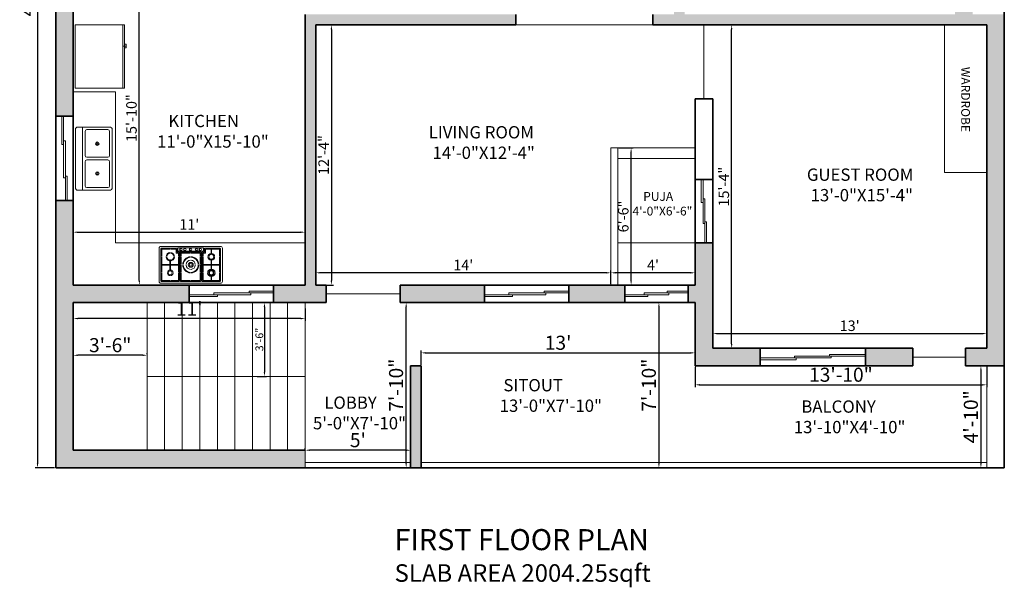
# Model space of a CAD drawing. Units: inches. Extents: x 3491 to 6898, y 1360 to 2019.
# Tile 8 of 9: x 6321 to 6882, y 1360 to 1683. Entities that reach past the tile are written whole.
import ezdxf

# ---------------------------------------------------------------- set-up
doc = ezdxf.new("R2010")
doc.units = ezdxf.units.IN
for name, color, linetype, lineweight in [('A-ANNO-DIMS', 2, 'Continuous', 18), ('A-ANNO-TEXT', 7, 'Continuous', 18), ('A-ANNO-TITL', 7, 'Continuous', 30), ('A-AREA-IDEN', 7, 'Continuous', 18), ('A-DOOR', 4, 'Continuous', 18), ('A-EQPM', 8, 'Continuous', 18), ('A-FLOR-CASE', 8, 'Continuous', 18), ('A-FLOR-FIXT', 8, 'Continuous', 18), ('A-FLOR-RAL', 7, 'Continuous', 18), ('A-FLOR-STRS', 7, 'Continuous', 18), ('A-GLAZ', 5, 'Continuous', 18), ('A-WALL', 7, 'Continuous', 35), ('A-WALL-PATT', 8, 'Continuous', 13)]:
    doc.layers.add(name, color=color, linetype=linetype, lineweight=lineweight)
doc.layers.add('A-WALL-OPEN', color=251, linetype='Continuous', lineweight=13, true_color=0x636466)
doc.styles.get("Standard").update_dxf_attribs({"font": 'arial.ttf'})
doc.dimstyles.new('ISO-25', dxfattribs={"dimtxt": 8, "dimasz": 2.5, "dimexe": 1.25, "dimexo": 0.625, "dimtad": 1, "dimdec": 1, "dimlunit": 3, "dimtxsty": 'Standard', "dimcen": 2.5, "dimclrt": 1, "dimadec": 0, "dimazin": 0, "dimtfac": 1, "dimtdec": 1, "dimtmove": 0, "dimatfit": 3, "dimfxl": 1, "dimarcsym": 0})

# ---------------------------------------------------------------- blocks, each defined once
blk = doc.blocks.new('*D35')
at = {"layer": 'A-ANNO-DIMS', "color": 0, "lineweight": -2, "transparency": 16777216}
for p, q in [((6341.16, 1972.37), (6330.15, 1972.37)), ((6331.4, 1969.87), (6331.4, 1430.87)), ((6341.16, 1428.37), (6330.15, 1428.37))]:
    blk.add_line(p, q, dxfattribs=at)
at = {"layer": 'A-ANNO-DIMS', "color": 0, "transparency": 16777216}
for points in [[(6330.99, 1969.87), (6331.82, 1969.87), (6331.4, 1972.37)], [(6330.99, 1430.87), (6331.82, 1430.87), (6331.4, 1428.37)]]:
    blk.add_solid(points, dxfattribs=at)
at = {"layer": 'Defpoints', "color": 0, "transparency": 16777216}
for p in [(6341.78, 1972.37), (6331.4, 1428.37), (6341.78, 1428.37)]:
    blk.add_point(p, dxfattribs=at)
at = {"layer": 'A-ANNO-DIMS', "color": 0, "transparency": 16777216, "insert": (6326.71, 1700.37), "char_height": 8, "attachment_point": 5, "rotation": 90}
blk.add_mtext('45\'-4"', dxfattribs=at)
blk = doc.blocks.new('*D36')
at = {"layer": 'A-ANNO-DIMS', "color": 0, "lineweight": -2, "transparency": 16777216}
for p, q in [((6351.78, 1493.03), (6351.78, 1493.65)), ((6391.28, 1492.4), (6354.28, 1492.4)), ((6393.78, 1493.03), (6393.78, 1493.65))]:
    blk.add_line(p, q, dxfattribs=at)
at = {"layer": 'A-ANNO-DIMS', "color": 0, "transparency": 16777216}
for points in [[(6354.28, 1492.82), (6354.28, 1491.99), (6351.78, 1492.4)], [(6391.28, 1492.82), (6391.28, 1491.99), (6393.78, 1492.4)]]:
    blk.add_solid(points, dxfattribs=at)
at = {"layer": 'Defpoints', "color": 0, "transparency": 16777216}
for p in [(6351.78, 1492.4), (6351.78, 1492.4), (6393.78, 1492.4)]:
    blk.add_point(p, dxfattribs=at)
at = {"layer": 'A-ANNO-DIMS', "color": 0, "transparency": 16777216, "insert": (6372.78, 1497.12), "char_height": 8, "attachment_point": 5}
blk.add_mtext('3\'-6"', dxfattribs=at)
blk = doc.blocks.new('*D30')
at = {"layer": 'A-ANNO-DIMS', "color": 0, "lineweight": -2, "transparency": 16777216}
for p, q in [((6456.5, 1522.37), (6461.84, 1522.37)), ((6460.59, 1519.87), (6460.59, 1482.87)), ((6456.5, 1480.37), (6461.84, 1480.37))]:
    blk.add_line(p, q, dxfattribs=at)
at = {"layer": 'A-ANNO-DIMS', "color": 0, "transparency": 16777216}
for points in [[(6460.17, 1519.87), (6461.01, 1519.87), (6460.59, 1522.37)], [(6460.17, 1482.87), (6461.01, 1482.87), (6460.59, 1480.37)]]:
    blk.add_solid(points, dxfattribs=at)
at = {"layer": 'Defpoints', "color": 0, "transparency": 16777216}
for p in [(6455.87, 1522.37), (6455.87, 1480.37), (6460.59, 1480.37)]:
    blk.add_point(p, dxfattribs=at)
at = {"layer": 'A-ANNO-DIMS', "color": 0, "transparency": 16777216, "insert": (6457.69, 1501.37), "char_height": 8, "attachment_point": 5, "rotation": 90}
blk.add_mtext('{\\H0.55556x;3\'-6"}', dxfattribs=at)
blk = doc.blocks.new('STOVE')
for p, q in [((11.85, 19.7), (11.55, 19.7)), ((11.55, 16.92), (11.55, 19.7)), ((11.85, 16.92), (11.55, 16.92)), ((11.85, 16.92), (11.85, 19.7)), ((-11.85, 13.73), (-11.85, 7.62)), ((-11.85, 13.73), (-11.55, 13.73)), ((-11.55, 13.73), (-11.55, 7.62)), ((11.85, 13.23), (11.55, 13.23)), ((11.55, 13.23), (11.55, 7.57)), ((11.85, 13.23), (11.85, 7.57)), ((-11.85, 10.75), (-16.4, 10.75)), ((-11.85, 10.25), (-16.4, 10.25)), ((-11.85, 7.62), (-11.55, 7.62)), ((-7, 10.75), (-11.55, 10.75)), ((-7, 10.25), (-11.55, 10.25)), ((7, 10.75), (11.55, 10.75)), ((7, 10.25), (11.55, 10.25)), ((11.85, 7.57), (11.55, 7.57)), ((11.85, 10.75), (16.4, 10.75)), ((11.85, 10.25), (16.4, 10.25)), ((-7, 3.9), (-8.4, 3.9)), ((-7.8, 3.3), (-7.8, 1)), ((-6.4, 3.3), (-7.8, 3.3)), ((7.3, 2.8), (-7.3, 2.8)), ((-7.3, 2.8), (-7.3, 0.8)), ((7.3, 0.8), (-7.3, 0.8)), ((-5.4, 3.9), (-6, 3.9)), ((-5.4, 3.9), (-0.15, 3.9)), ((0.15, 3.9), (5.4, 3.9)), ((6.4, 3.3), (7.8, 3.3)), ((7, 3.9), (8.4, 3.9)), ((7.3, 2.8), (7.3, 0.8)), ((7.8, 3.3), (7.8, 1)), ((8.4, 3.9), (8.4, 1.6)), ((11.85, 4.28), (11.55, 4.28)), ((11.55, 4.28), (11.55, 1.3)), ((11.85, 1.3), (11.55, 1.3)), ((11.85, 4.28), (11.85, 1.3))]:
    blk.add_line(p, q)
for points in [[(-17, 21), (17, 21, -0.414214), (18, 20), (18, 1, -0.414214), (17, 0), (-17, 0, -0.414214), (-18, 1), (-18, 20, -0.414214)], [(6, 3.3), (-6, 3.3), (-6, 19.4, -0.414214), (-5.4, 20), (5.4, 20, -0.414214), (6, 19.4)]]:
    blk.add_lwpolyline(points, format="xyb", close=True)
for points in [[(-7.8, 1), (-16.4, 1, -0.414214), (-17, 1.6), (-17, 19.4, -0.414214), (-16.4, 20), (-7, 20, -0.414214), (-6.4, 19.4), (-6.4, 3.3)], [(6.4, 19.4, -0.414214), (7, 20), (16.4, 20, -0.414214), (17, 19.4), (17, 1.6, -0.414214), (16.4, 1), (7.8, 1)]]:
    blk.add_lwpolyline(points, format="xyb")
for points in [[(-16.4, 15.22), (-16.4, 19.4), (-11.85, 19.4)], [(-11.55, 19.4), (-7, 19.4), (-7, 15.22)], [(-5.4, 15.22), (-5.4, 19.4), (-0.15, 19.4)], [(0.15, 19.4), (5.4, 19.4), (5.4, 15.22)], [(6.4, 3.3), (6.4, 19.4)], [(7, 15.22), (7, 19.4), (11.55, 19.4)], [(11.85, 19.4), (16.4, 19.4), (16.4, 15.22)], [(-16.4, 6.08), (-16.4, 14.92)], [(-7, 14.92), (-7, 6.08)], [(-5.4, 10.65), (-5.4, 14.92)], [(5.4, 14.92), (5.4, 10.65)], [(7, 6.08), (7, 14.92)], [(16.4, 14.92), (16.4, 6.08)], [(-11.85, 1.6), (-16.4, 1.6), (-16.4, 5.77)], [(-7, 5.77), (-7, 3.9)], [(-5.4, 6.08), (-5.4, 10.35)], [(-5.4, 3.9), (-5.4, 5.77)], [(5.4, 10.35), (5.4, 6.08)], [(5.4, 5.77), (5.4, 3.9)], [(7, 3.9), (7, 5.77)], [(16.4, 5.77), (16.4, 1.6), (11.85, 1.6)], [(-8.4, 3.9), (-8.4, 1.6), (-11.55, 1.6)], [(11.55, 1.6), (8.4, 1.6)]]:
    blk.add_lwpolyline(points)
for centre, radius in [((-11.7, 15.07), 1.1), ((0, 10.5), 1.4), ((0, 10.5), 0.8), ((11.7, 15.07), 1.6), ((11.7, 15.07), 1.1), ((11.7, 5.93), 1.4), ((-5.49, 1.8), 0.6), ((-3.3, 1.8), 0.6), ((0, 1.8), 0.6), ((3.39, 1.8), 0.6), ((5.57, 1.8), 0.6)]:
    blk.add_circle(centre, radius)
for centre, radius, start, end in [((11.7, 15.07), 2.1, 94.096, 175.904), ((11.7, 15.07), 2.1, 4.096, 85.904), ((-11.7, 15.07), 1.6, 95.3794, 174.6206), ((-11.7, 15.07), 1.6, 185.3794, 264.6206), ((-11.7, 15.07), 1.6, 5.3794, 84.6206), ((-11.7, 15.07), 1.6, 275.3794, 354.6206), ((0, 10.5), 4.6, 91.8687, 178.1313), ((0, 10.5), 4.3, 91.9991, 178.0009), ((0, 10.5), 2.6, 93.3074, 176.6926), ((0, 10.5), 4.6, 1.8687, 88.1313), ((0, 10.5), 4.3, 1.9991, 88.0009), ((0, 10.5), 2.6, 3.3074, 86.6926), ((11.7, 15.07), 2.1, 184.096, 265.904), ((11.7, 15.07), 2.1, 274.096, 355.904), ((-11.7, 5.93), 2.4, 93.5833, 176.4167), ((-11.7, 5.93), 2.4, 183.5833, 266.4167), ((-11.7, 5.93), 2, 94.3012, 175.6988), ((-11.7, 5.93), 2, 184.3012, 265.6988), ((-11.7, 5.93), 2.4, 3.5833, 86.4167), ((-11.7, 5.93), 2, 4.3012, 85.6988), ((-11.7, 5.93), 2.4, 273.5833, 356.4167), ((-11.7, 5.93), 2, 274.3012, 355.6988), ((0, 10.5), 4.6, 181.8687, 268.1313), ((0, 10.5), 4.3, 181.9991, 268.0009), ((0, 10.5), 2.6, 183.3074, 266.6926), ((0, 10.5), 4.6, 271.8687, 358.1313), ((0, 10.5), 4.3, 271.9991, 358.0009), ((0, 10.5), 2.6, 273.3074, 356.6926), ((11.7, 5.93), 1.9, 94.5281, 175.4719), ((11.7, 5.93), 1.9, 184.5281, 265.4719), ((11.7, 5.93), 1.9, 4.5281, 85.4719), ((11.7, 5.93), 1.9, 274.5281, 355.4719), ((-5.49, 1.8), 0.846, 89.9979, 270), ((-3.3, 1.8), 0.846, 89.9979, 270), ((0, 1.8), 0.846, 89.9979, 270), ((3.39, 1.8), 0.846, 89.9979, 270), ((5.57, 1.8), 0.846, 89.9979, 270)]:
    blk.add_arc(centre, radius, start, end)
blk = doc.blocks.new('Sink-double - 36 in top')
for p, q in [((-18, -4), (18, -4)), ((-0.75, -18.5), (-0.75, -6.5)), ((0.75, -6.5), (0.75, -18.5))]:
    blk.add_line(p, q)
for points in [[(-16.5, 0), (16.5, 0)], [(-18, -19.5), (-18, -1.5)], [(-15.5, -5.5), (-1.75, -5.5)], [(1.75, -5.5), (15.5, -5.5)], [(18, -1.5), (18, -19.5)], [(-16.5, -18.5), (-16.5, -6.5)], [(16.5, -6.5), (16.5, -18.5)], [(16.5, -21), (-16.5, -21)], [(-1.75, -19.5), (-15.5, -19.5)], [(15.5, -19.5), (1.75, -19.5)]]:
    blk.add_lwpolyline(points)
for centre, radius in [((-8.5, -12.5), 1), ((-8.5, -12.5), 0.5), ((8.5, -12.5), 1), ((8.5, -12.5), 0.5)]:
    blk.add_circle(centre, radius)
for centre, radius, start, end in [((-16.5, -1.5), 1.5, 90, 180), ((16.5, -1.5), 1.5, 0, 90), ((-15.5, -6.5), 1, 90, 180), ((-1.75, -6.5), 1, 0, 90), ((1.75, -6.5), 1, 90, 180), ((15.5, -6.5), 1, 0, 90), ((-16.5, -19.5), 1.5, 180, 270), ((-15.5, -18.5), 1, 180, 270), ((-1.75, -18.5), 1, 270, 0), ((1.75, -18.5), 1, 180, 270), ((15.5, -18.5), 1, 270, 0), ((16.5, -19.5), 1.5, 270, 0)]:
    blk.add_arc(centre, radius, start, end)
blk = doc.blocks.new('Refrigerator-2 door - 36 in top')
for p, q in [((0, -26.999999), (36, -26.999999)), ((11, -27.999999), (11, -28.999999)), ((12, -26.999999), (12, -28.999999)), ((13, -28.999999), (13, -27.999999)), ((11, -28.999999), (13, -28.999999))]:
    blk.add_line(p, q)
blk.add_lwpolyline([(0, -27.999999), (0, 0), (36, 0), (36, -27.999999)], close=True)
blk = doc.blocks.new('*D37')
at = {"layer": 'A-ANNO-DIMS', "color": 0, "lineweight": -2, "transparency": 16777216}
for p, q in [((6351.78, 1521.74), (6351.78, 1512.03)), ((6483.78, 1518.98), (6483.78, 1512.03)), ((6481.28, 1513.28), (6354.28, 1513.28))]:
    blk.add_line(p, q, dxfattribs=at)
at = {"layer": 'A-ANNO-DIMS', "color": 0, "transparency": 16777216}
for points in [[(6354.28, 1513.7), (6354.28, 1512.87), (6351.78, 1513.28)], [(6481.28, 1513.7), (6481.28, 1512.87), (6483.78, 1513.28)]]:
    blk.add_solid(points, dxfattribs=at)
at = {"layer": 'Defpoints', "color": 0, "transparency": 16777216}
for p in [(6351.78, 1522.37), (6483.78, 1519.61), (6351.78, 1513.28)]:
    blk.add_point(p, dxfattribs=at)
at = {"layer": 'A-ANNO-DIMS', "color": 0, "transparency": 16777216, "insert": (6417.78, 1517.92), "char_height": 8, "attachment_point": 5}
blk.add_mtext("11'", dxfattribs=at)
blk = doc.blocks.new('*D40')
at = {"layer": 'A-ANNO-DIMS', "color": 0, "lineweight": -2, "transparency": 16777216}
for p, q in [((6705.78, 1485.74), (6705.78, 1474.33)), ((6871.78, 1485.74), (6871.78, 1474.33)), ((6708.28, 1475.58), (6869.28, 1475.58))]:
    blk.add_line(p, q, dxfattribs=at)
at = {"layer": 'A-ANNO-DIMS', "color": 0, "transparency": 16777216}
for points in [[(6708.28, 1476), (6708.28, 1475.16), (6705.78, 1475.58)], [(6869.28, 1476), (6869.28, 1475.16), (6871.78, 1475.58)]]:
    blk.add_solid(points, dxfattribs=at)
at = {"layer": 'Defpoints', "color": 0, "transparency": 16777216}
for p in [(6705.78, 1486.37), (6871.78, 1486.37), (6871.78, 1475.58)]:
    blk.add_point(p, dxfattribs=at)
at = {"layer": 'A-ANNO-DIMS', "color": 0, "transparency": 16777216, "insert": (6788.78, 1480.29), "char_height": 8, "attachment_point": 5}
blk.add_mtext('13\'-10"', dxfattribs=at)
blk = doc.blocks.new('*D41')
at = {"layer": 'A-ANNO-DIMS', "color": 0, "lineweight": -2, "transparency": 16777216}
for p, q in [((6871.16, 1486.37), (6867.23, 1486.37)), ((6868.48, 1483.87), (6868.48, 1430.87)), ((6871.16, 1428.37), (6867.23, 1428.37))]:
    blk.add_line(p, q, dxfattribs=at)
at = {"layer": 'A-ANNO-DIMS', "color": 0, "transparency": 16777216}
for points in [[(6868.06, 1483.87), (6868.9, 1483.87), (6868.48, 1486.37)], [(6868.06, 1430.87), (6868.9, 1430.87), (6868.48, 1428.37)]]:
    blk.add_solid(points, dxfattribs=at)
at = {"layer": 'Defpoints', "color": 0, "transparency": 16777216}
for p in [(6871.78, 1486.37), (6868.48, 1428.37), (6871.78, 1428.37)]:
    blk.add_point(p, dxfattribs=at)
at = {"layer": 'A-ANNO-DIMS', "color": 0, "transparency": 16777216, "insert": (6863.77, 1457.37), "char_height": 8, "attachment_point": 5, "rotation": 90}
blk.add_mtext('4\'-10"', dxfattribs=at)
blk = doc.blocks.new('*D42')
at = {"layer": 'A-ANNO-DIMS', "color": 0, "lineweight": -2, "transparency": 16777216}
for p, q in [((6549.78, 1486.99), (6549.78, 1495.02)), ((6552.28, 1493.77), (6703.28, 1493.77)), ((6705.78, 1486.99), (6705.78, 1495.02))]:
    blk.add_line(p, q, dxfattribs=at)
at = {"layer": 'A-ANNO-DIMS', "color": 0, "transparency": 16777216}
for points in [[(6552.28, 1494.19), (6552.28, 1493.35), (6549.78, 1493.77)], [(6703.28, 1494.19), (6703.28, 1493.35), (6705.78, 1493.77)]]:
    blk.add_solid(points, dxfattribs=at)
at = {"layer": 'Defpoints', "color": 0, "transparency": 16777216}
for p in [(6705.78, 1493.77), (6549.78, 1486.37), (6705.78, 1486.37)]:
    blk.add_point(p, dxfattribs=at)
at = {"layer": 'A-ANNO-DIMS', "color": 0, "transparency": 16777216, "insert": (6627.78, 1498.48), "char_height": 8, "attachment_point": 5}
blk.add_mtext("13'", dxfattribs=at)
blk = doc.blocks.new('*D43')
at = {"layer": 'A-ANNO-DIMS', "color": 0, "lineweight": -2, "transparency": 16777216}
for p, q in [((6685.16, 1519.87), (6685.16, 1430.87)), ((6685.78, 1522.37), (6686.41, 1522.37)), ((6685.78, 1428.37), (6686.41, 1428.37))]:
    blk.add_line(p, q, dxfattribs=at)
at = {"layer": 'A-ANNO-DIMS', "color": 0, "transparency": 16777216}
for points in [[(6684.74, 1519.87), (6685.57, 1519.87), (6685.16, 1522.37)], [(6684.74, 1430.87), (6685.57, 1430.87), (6685.16, 1428.37)]]:
    blk.add_solid(points, dxfattribs=at)
at = {"layer": 'Defpoints', "color": 0, "transparency": 16777216}
for p in [(6685.16, 1522.37), (6685.16, 1428.37), (6685.16, 1428.37)]:
    blk.add_point(p, dxfattribs=at)
at = {"layer": 'A-ANNO-DIMS', "color": 0, "transparency": 16777216, "insert": (6680.45, 1475.37), "char_height": 8, "attachment_point": 5, "rotation": 90}
blk.add_mtext('7\'-10"', dxfattribs=at)
blk = doc.blocks.new('*D38')
at = {"layer": 'A-ANNO-DIMS', "color": 0, "lineweight": -2, "transparency": 16777216}
for p, q in [((6538.41, 1522.37), (6542.52, 1522.37)), ((6541.27, 1430.87), (6541.27, 1519.87)), ((6534.73, 1428.37), (6542.52, 1428.37))]:
    blk.add_line(p, q, dxfattribs=at)
at = {"layer": 'A-ANNO-DIMS', "color": 0, "transparency": 16777216}
for points in [[(6540.86, 1519.87), (6541.69, 1519.87), (6541.27, 1522.37)], [(6540.86, 1430.87), (6541.69, 1430.87), (6541.27, 1428.37)]]:
    blk.add_solid(points, dxfattribs=at)
at = {"layer": 'Defpoints', "color": 0, "transparency": 16777216}
for p in [(6537.78, 1522.37), (6541.27, 1522.37), (6534.1, 1428.37)]:
    blk.add_point(p, dxfattribs=at)
at = {"layer": 'A-ANNO-DIMS', "color": 0, "transparency": 16777216, "insert": (6536.56, 1475.37), "char_height": 8, "attachment_point": 5, "rotation": 90}
blk.add_mtext('7\'-10"', dxfattribs=at)
blk = doc.blocks.new('*D39')
at = {"layer": 'A-ANNO-DIMS', "color": 0, "lineweight": -2, "transparency": 16777216}
for p, q in [((6483.78, 1438.99), (6483.78, 1439.62)), ((6541.28, 1438.37), (6486.28, 1438.37)), ((6543.78, 1438.46), (6543.78, 1439.62))]:
    blk.add_line(p, q, dxfattribs=at)
at = {"layer": 'A-ANNO-DIMS', "color": 0, "transparency": 16777216}
for points in [[(6486.28, 1438.78), (6486.28, 1437.95), (6483.78, 1438.37)], [(6541.28, 1438.78), (6541.28, 1437.95), (6543.78, 1438.37)]]:
    blk.add_solid(points, dxfattribs=at)
at = {"layer": 'Defpoints', "color": 0, "transparency": 16777216}
for p in [(6483.78, 1438.37), (6483.78, 1438.37), (6543.78, 1437.84)]:
    blk.add_point(p, dxfattribs=at)
at = {"layer": 'A-ANNO-DIMS', "color": 0, "transparency": 16777216, "insert": (6513.78, 1443.06), "char_height": 8, "attachment_point": 5}
blk.add_mtext("5'", dxfattribs=at)
blk = doc.blocks.new('*D75')
at = {"layer": 'A-ANNO-DIMS', "color": 0, "lineweight": -2, "transparency": 16777216}
for p, q in [((6351.78, 1532.99), (6351.78, 1563.69)), ((6354.28, 1562.44), (6481.28, 1562.44)), ((6483.78, 1532.99), (6483.78, 1563.69))]:
    blk.add_line(p, q, dxfattribs=at)
at = {"layer": 'A-ANNO-DIMS', "color": 0, "transparency": 16777216}
for points in [[(6354.28, 1562.85), (6354.28, 1562.02), (6351.78, 1562.44)], [(6481.28, 1562.85), (6481.28, 1562.02), (6483.78, 1562.44)]]:
    blk.add_solid(points, dxfattribs=at)
at = {"layer": 'Defpoints', "color": 0, "transparency": 16777216}
for p in [(6483.78, 1562.44), (6351.78, 1532.37), (6483.78, 1532.37)]:
    blk.add_point(p, dxfattribs=at)
at = {"layer": 'A-ANNO-DIMS', "color": 0, "transparency": 16777216, "insert": (6417.78, 1566.07), "char_height": 6, "attachment_point": 5}
blk.add_mtext("11'", dxfattribs=at)
blk = doc.blocks.new('*D76')
at = {"layer": 'A-ANNO-DIMS', "color": 0, "lineweight": -2, "transparency": 16777216}
for p, q in [((6352.41, 1722.37), (6390.61, 1722.37)), ((6389.36, 1534.87), (6389.36, 1719.87)), ((6352.41, 1532.37), (6390.61, 1532.37))]:
    blk.add_line(p, q, dxfattribs=at)
at = {"layer": 'A-ANNO-DIMS', "color": 0, "transparency": 16777216}
for points in [[(6388.94, 1719.87), (6389.78, 1719.87), (6389.36, 1722.37)], [(6388.94, 1534.87), (6389.78, 1534.87), (6389.36, 1532.37)]]:
    blk.add_solid(points, dxfattribs=at)
at = {"layer": 'Defpoints', "color": 0, "transparency": 16777216}
for p in [(6351.78, 1722.37), (6389.36, 1722.37), (6351.78, 1532.37)]:
    blk.add_point(p, dxfattribs=at)
at = {"layer": 'A-ANNO-DIMS', "color": 0, "transparency": 16777216, "insert": (6385.67, 1627.37), "char_height": 6, "attachment_point": 5, "rotation": 90}
blk.add_mtext('15\'-10"', dxfattribs=at)
blk = doc.blocks.new('*D77')
at = {"layer": 'A-ANNO-DIMS', "color": 0, "lineweight": -2, "transparency": 16777216}
for p, q in [((6490.41, 1680.37), (6499.96, 1680.37)), ((6498.71, 1677.87), (6498.71, 1534.87)), ((6490.41, 1532.37), (6499.96, 1532.37))]:
    blk.add_line(p, q, dxfattribs=at)
at = {"layer": 'A-ANNO-DIMS', "color": 0, "transparency": 16777216}
for points in [[(6498.29, 1677.87), (6499.13, 1677.87), (6498.71, 1680.37)], [(6498.29, 1534.87), (6499.13, 1534.87), (6498.71, 1532.37)]]:
    blk.add_solid(points, dxfattribs=at)
at = {"layer": 'Defpoints', "color": 0, "transparency": 16777216}
for p in [(6489.78, 1680.37), (6489.78, 1532.37), (6498.71, 1532.37)]:
    blk.add_point(p, dxfattribs=at)
at = {"layer": 'A-ANNO-DIMS', "color": 0, "transparency": 16777216, "insert": (6495.07, 1606.37), "char_height": 6, "attachment_point": 5, "rotation": 90}
blk.add_mtext('12\'-4"', dxfattribs=at)
blk = doc.blocks.new('*D78')
at = {"layer": 'A-ANNO-DIMS', "color": 0, "lineweight": -2, "transparency": 16777216}
for p, q in [((6489.78, 1532.99), (6489.78, 1540.59)), ((6655.28, 1539.34), (6492.28, 1539.34)), ((6657.78, 1532.99), (6657.78, 1540.59))]:
    blk.add_line(p, q, dxfattribs=at)
at = {"layer": 'A-ANNO-DIMS', "color": 0, "transparency": 16777216}
for points in [[(6492.28, 1539.75), (6492.28, 1538.92), (6489.78, 1539.34)], [(6655.28, 1539.75), (6655.28, 1538.92), (6657.78, 1539.34)]]:
    blk.add_solid(points, dxfattribs=at)
at = {"layer": 'Defpoints', "color": 0, "transparency": 16777216}
for p in [(6489.78, 1539.34), (6489.78, 1532.37), (6657.78, 1532.37)]:
    blk.add_point(p, dxfattribs=at)
at = {"layer": 'A-ANNO-DIMS', "color": 0, "transparency": 16777216, "insert": (6573.78, 1542.98), "char_height": 6, "attachment_point": 5}
blk.add_mtext("14'", dxfattribs=at)
blk = doc.blocks.new('*D79')
at = {"layer": 'A-ANNO-DIMS', "color": 0, "lineweight": -2, "transparency": 16777216}
for p, q in [((6657.78, 1532.99), (6657.78, 1540.59)), ((6703.28, 1539.34), (6660.28, 1539.34)), ((6705.78, 1532.99), (6705.78, 1540.59))]:
    blk.add_line(p, q, dxfattribs=at)
at = {"layer": 'A-ANNO-DIMS', "color": 0, "transparency": 16777216}
for points in [[(6660.28, 1539.75), (6660.28, 1538.92), (6657.78, 1539.34)], [(6703.28, 1539.75), (6703.28, 1538.92), (6705.78, 1539.34)]]:
    blk.add_solid(points, dxfattribs=at)
at = {"layer": 'Defpoints', "color": 0, "transparency": 16777216}
for p in [(6657.78, 1539.34), (6657.78, 1532.37), (6705.78, 1532.37)]:
    blk.add_point(p, dxfattribs=at)
at = {"layer": 'A-ANNO-DIMS', "color": 0, "transparency": 16777216, "insert": (6681.78, 1542.96), "char_height": 6, "attachment_point": 5}
blk.add_mtext("4'", dxfattribs=at)
blk = doc.blocks.new('*D80')
at = {"layer": 'A-ANNO-DIMS', "color": 0, "lineweight": -2, "transparency": 16777216}
for p, q in [((6662.41, 1610.37), (6670.57, 1610.37)), ((6669.32, 1534.87), (6669.32, 1607.87)), ((6662.41, 1532.37), (6670.57, 1532.37))]:
    blk.add_line(p, q, dxfattribs=at)
at = {"layer": 'A-ANNO-DIMS', "color": 0, "transparency": 16777216}
for points in [[(6668.9, 1607.87), (6669.74, 1607.87), (6669.32, 1610.37)], [(6668.9, 1534.87), (6669.74, 1534.87), (6669.32, 1532.37)]]:
    blk.add_solid(points, dxfattribs=at)
at = {"layer": 'Defpoints', "color": 0, "transparency": 16777216}
for p in [(6661.78, 1610.37), (6669.32, 1610.37), (6661.78, 1532.37)]:
    blk.add_point(p, dxfattribs=at)
at = {"layer": 'A-ANNO-DIMS', "color": 0, "transparency": 16777216, "insert": (6665.63, 1571.37), "char_height": 6, "attachment_point": 5, "rotation": 90}
blk.add_mtext('6\'-6"', dxfattribs=at)
blk = doc.blocks.new('*D81')
at = {"layer": 'A-ANNO-DIMS', "color": 0, "lineweight": -2, "transparency": 16777216}
for p, q in [((6715.78, 1496.99), (6715.78, 1505.99)), ((6718.28, 1504.74), (6869.28, 1504.74)), ((6871.78, 1496.99), (6871.78, 1505.99))]:
    blk.add_line(p, q, dxfattribs=at)
at = {"layer": 'A-ANNO-DIMS', "color": 0, "transparency": 16777216}
for points in [[(6718.28, 1505.15), (6718.28, 1504.32), (6715.78, 1504.74)], [(6869.28, 1505.15), (6869.28, 1504.32), (6871.78, 1504.74)]]:
    blk.add_solid(points, dxfattribs=at)
at = {"layer": 'Defpoints', "color": 0, "transparency": 16777216}
for p in [(6871.78, 1504.74), (6715.78, 1496.37), (6871.78, 1496.37)]:
    blk.add_point(p, dxfattribs=at)
at = {"layer": 'A-ANNO-DIMS', "color": 0, "transparency": 16777216, "insert": (6793.78, 1508.43), "char_height": 6, "attachment_point": 5}
blk.add_mtext("13'", dxfattribs=at)
blk = doc.blocks.new('*D82')
at = {"layer": 'A-ANNO-DIMS', "color": 0, "lineweight": -2, "transparency": 16777216}
for p, q in [((6716.41, 1680.37), (6727.81, 1680.37)), ((6726.56, 1498.87), (6726.56, 1677.87)), ((6716.41, 1496.37), (6727.81, 1496.37))]:
    blk.add_line(p, q, dxfattribs=at)
at = {"layer": 'A-ANNO-DIMS', "color": 0, "transparency": 16777216}
for points in [[(6726.15, 1677.87), (6726.98, 1677.87), (6726.56, 1680.37)], [(6726.15, 1498.87), (6726.98, 1498.87), (6726.56, 1496.37)]]:
    blk.add_solid(points, dxfattribs=at)
at = {"layer": 'Defpoints', "color": 0, "transparency": 16777216}
for p in [(6715.78, 1680.37), (6726.56, 1680.37), (6715.78, 1496.37)]:
    blk.add_point(p, dxfattribs=at)
at = {"layer": 'A-ANNO-DIMS', "color": 0, "transparency": 16777216, "insert": (6722.87, 1588.37), "char_height": 6, "attachment_point": 5, "rotation": 90}
blk.add_mtext('15\'-4"', dxfattribs=at)
blk = doc.blocks.new('WIN-SLIDER-48IN')
for p, q in [((35, 1), (0, 1)), ((48, 2), (14, 2)), ((14, 2), (14, 1)), ((16, 1), (16, 0)), ((34, 3), (34, 2)), ((48, 3), (34, 3)), ((35, 2), (35, 1)), ((16, 0), (0, 0))]:
    blk.add_line(p, q)
blk = doc.blocks.new('WIN-SLIDER-36IN')
for p, q in [((25, 1), (0, 1)), ((13, 0), (0, 0)), ((36, 2), (11, 2)), ((11, 2), (11, 1)), ((13, 1), (13, 0)), ((24, 3), (24, 2)), ((36, 3), (24, 3)), ((25, 2), (25, 1))]:
    blk.add_line(p, q)
blk = doc.blocks.new('WIN-SLIDER-60IN')
for p, q in [((0, 39.5), (0, 60)), ((1, 19.5), (1, 60)), ((1, 39.5), (0, 39.5)), ((2, 40.5), (1, 40.5)), ((2, 0), (2, 40.5)), ((2, 19.5), (1, 19.5)), ((3, 20.5), (2, 20.5)), ((3, 0), (3, 20.5))]:
    blk.add_line(p, q)
blk = doc.blocks.new('STAIR-RETURN-FLIGHT')
for p, q in [((0, 84), (0, 0)), ((10, 84), (10, 0)), ((20, 84), (20, 0)), ((30, 84), (30, 0)), ((40, 84), (40, 0)), ((50, 84), (50, 0)), ((60, 84), (60, 0)), ((70, 84), (70, 0)), ((80, 84), (80, 0)), ((0, 42), (90, 42))]:
    blk.add_line(p, q)
blk = doc.blocks.new('COUNTER-KITCHEN-L')
for p, q in [((24, 86.04), (0, 86.04)), ((24, 86.04), (24, 0)), ((132, 0), (24, 0))]:
    blk.add_line(p, q)
blk = doc.blocks.new('PUJA-ALCOVE-48X78')
for p, q in [((0, 78), (0, 0)), ((48, 78), (0, 78)), ((4, 78), (4, 0)), ((48, 72), (4, 72)), ((48, 24), (4, 24))]:
    blk.add_line(p, q)
blk = doc.blocks.new('WARDROBE-84X24')
for q in [(0, 84), (24, 0)]:
    blk.add_line((24, 84), q)

msp = doc.modelspace()

# ---------------------------------------------------------------- hatches: boundary and pattern name
at = {"layer": 'A-WALL-PATT'}
h = msp.add_hatch(color=256, dxfattribs=at)
h.dxf.hatch_style = 1
h.paths.add_polyline_path([(6665.78, 1532.37), (6657.78, 1532.37), (6633.8, 1532.37), (6633.8, 1522.37), (6665.78, 1522.37)])
h.paths.add_polyline_path([(6715.78, 1556.37), (6705.78, 1556.37), (6705.78, 1532.37), (6701.78, 1532.37), (6701.78, 1522.37), (6705.78, 1522.37), (6705.78, 1486.37), (6742.76, 1486.37), (6742.76, 1496.37), (6715.78, 1496.37)], flags=17)
h.paths.add_polyline_path([(6585.8, 1532.37), (6537.78, 1532.37), (6537.78, 1522.37), (6585.8, 1522.37)], flags=17)
h.paths.add_polyline_path([(6829.78, 1496.37), (6802.76, 1496.37), (6802.76, 1486.37), (6829.78, 1486.37)], flags=17)
h.paths.add_polyline_path([(6881.78, 1686.37), (6863.78, 1686.37), (6863.78, 1719.37), (6853.78, 1719.37), (6853.78, 1686.37), (6699.78, 1686.37), (6699.78, 1776.37), (6693.78, 1776.37), (6693.78, 1686.37), (6681.78, 1686.37), (6681.78, 1680.37), (6871.78, 1680.37), (6871.78, 1496.37), (6859.78, 1496.37), (6859.78, 1486.37), (6881.78, 1486.37)])
h.paths.add_polyline_path([(6603.78, 1686.37), (6483.78, 1686.37), (6483.78, 1532.37), (6465.81, 1532.37), (6465.81, 1522.37), (6495.78, 1522.37), (6495.78, 1532.37), (6489.78, 1532.37), (6489.78, 1680.37), (6603.78, 1680.37)])
h.paths.add_polyline_path([(6351.78, 1722.37), (6429.78, 1722.37), (6429.78, 1782.37), (6423.78, 1782.37), (6423.78, 1728.37), (6351.78, 1728.37), (6351.78, 1770.37), (6341.78, 1770.37), (6341.78, 1628.4), (6351.78, 1628.4)])
h.paths.add_polyline_path([(6351.78, 1580.4), (6341.78, 1580.4), (6341.78, 1428.37), (6483.78, 1428.37), (6483.78, 1438.37), (6351.78, 1438.37), (6351.78, 1522.37), (6417.81, 1522.37), (6417.81, 1532.37), (6351.78, 1532.37)])
h.paths.add_polyline_path([(6549.78, 1486.37), (6543.78, 1486.37), (6543.78, 1428.37), (6549.78, 1428.37)])
h.paths.add_polyline_path([(6863.78, 1857.37), (6853.78, 1857.37), (6853.78, 1818.37), (6693.78, 1818.37), (6693.78, 1812.37), (6853.78, 1812.37), (6853.78, 1779.37), (6863.78, 1779.37)])
h.paths.add_polyline_path([(6657.78, 1872.37), (6651.78, 1872.37), (6651.78, 1818.37), (6591.78, 1818.37), (6591.78, 1902.37), (6609.78, 1902.37), (6609.78, 1908.37), (6567.78, 1908.37), (6567.78, 1902.37), (6585.78, 1902.37), (6585.78, 1818.37), (6525.78, 1818.37), (6525.78, 1872.37), (6519.78, 1872.37), (6519.78, 1812.37), (6657.78, 1812.37)])
h.paths.add_polyline_path([(6351.78, 1857.37), (6341.78, 1857.37), (6341.78, 1794.37), (6351.78, 1794.37), (6351.78, 1812.37), (6483.78, 1812.37), (6483.78, 1818.37), (6351.78, 1818.37)])
h.paths.add_polyline_path([(6351.78, 1962.37), (6519.78, 1962.37), (6519.78, 1938.37), (6525.78, 1938.37), (6525.78, 1962.37), (6651.78, 1962.37), (6651.78, 1938.37), (6657.78, 1938.37), (6657.78, 1962.37), (6853.78, 1962.37), (6853.78, 1923.37), (6863.78, 1923.37), (6863.78, 1972.37), (6341.78, 1972.37), (6341.78, 1923.37), (6351.78, 1923.37)])
h.paths.add_polyline_path([(6657.78, 1908.37), (6633.78, 1908.37), (6633.78, 1902.37), (6657.78, 1902.37)], flags=17)
h.paths.add_polyline_path([(6543.78, 1908.37), (6519.78, 1908.37), (6519.78, 1902.37), (6543.78, 1902.37)], flags=17)

# ---------------------------------------------------------------- linework, layer by layer
at = {"layer": 'A-DOOR'}
for p, q in [((6710.78, 1638.37), (6710.78, 1680.37)), ((6537.78, 1527.37), (6495.78, 1527.37)), ((6859.78, 1491.37), (6829.78, 1491.37))]:
    msp.add_line(p, q, dxfattribs=at)
at = {"layer": 'A-FLOR-RAL'}
for p, q in [((6871.78, 1486.37), (6871.78, 1428.37)), ((6483.78, 1431.37), (6543.78, 1431.37)), ((6549.78, 1431.37), (6871.78, 1431.37))]:
    msp.add_line(p, q, dxfattribs=at)
at = {"layer": 'A-FLOR-STRS'}
msp.add_line((6483.78, 1522.37), (6483.78, 1428.37), dxfattribs=at)
at = {"layer": 'A-WALL'}
for p, q in [((6341.78, 1972.37), (6341.78, 1428.37)), ((6881.78, 1428.37), (6881.78, 1972.37)), ((6351.78, 1722.37), (6351.78, 1532.37)), ((6483.78, 1686.37), (6483.78, 1532.37)), ((6603.78, 1686.37), (6603.78, 1680.37)), ((6681.78, 1686.37), (6681.78, 1680.37)), ((6603.78, 1680.37), (6489.78, 1680.37)), ((6489.78, 1680.37), (6489.78, 1532.37)), ((6871.78, 1680.37), (6681.78, 1680.37)), ((6871.78, 1496.37), (6871.78, 1680.37)), ((6715.78, 1638.37), (6705.78, 1638.37)), ((6705.78, 1638.37), (6705.78, 1532.37)), ((6715.78, 1638.37), (6715.78, 1496.37)), ((6351.78, 1628.4), (6341.78, 1628.4)), ((6715.78, 1592.37), (6705.78, 1592.37)), ((6351.78, 1580.4), (6341.78, 1580.4)), ((6715.78, 1556.37), (6705.78, 1556.37)), ((6483.78, 1532.37), (6351.78, 1532.37)), ((6417.81, 1532.37), (6417.81, 1522.37)), ((6465.81, 1532.37), (6465.81, 1522.37)), ((6495.78, 1532.37), (6489.78, 1532.37)), ((6495.78, 1532.37), (6495.78, 1522.37)), ((6657.78, 1532.37), (6537.78, 1532.37)), ((6537.78, 1532.37), (6537.78, 1522.37)), ((6585.8, 1532.37), (6585.8, 1522.37)), ((6633.8, 1532.37), (6633.8, 1522.37)), ((6705.78, 1532.37), (6657.78, 1532.37)), ((6665.78, 1532.37), (6665.78, 1522.37)), ((6701.78, 1532.37), (6701.78, 1522.37)), ((6495.78, 1522.37), (6351.78, 1522.37)), ((6351.78, 1522.37), (6351.78, 1438.37)), ((6705.78, 1522.37), (6537.78, 1522.37)), ((6705.78, 1522.37), (6705.78, 1486.37)), ((6829.78, 1496.37), (6715.78, 1496.37)), ((6742.76, 1486.37), (6742.76, 1496.37)), ((6802.76, 1486.37), (6802.76, 1496.37)), ((6829.78, 1486.37), (6829.78, 1496.37)), ((6871.78, 1496.37), (6859.78, 1496.37)), ((6859.78, 1486.37), (6859.78, 1496.37)), ((6549.78, 1486.37), (6543.78, 1486.37)), ((6543.78, 1486.37), (6543.78, 1428.37)), ((6549.78, 1486.37), (6549.78, 1428.37)), ((6829.78, 1486.37), (6705.78, 1486.37)), ((6881.78, 1486.37), (6859.78, 1486.37)), ((6351.78, 1438.37), (6483.78, 1438.37)), ((6341.78, 1428.37), (6881.78, 1428.37))]:
    msp.add_line(p, q, dxfattribs=at)
at = {"layer": 'A-WALL-OPEN'}
msp.add_line((6603.78, 1680.37), (6681.78, 1680.37), dxfattribs=at)

# ---------------------------------------------------------------- block references
at = {"layer": 'A-EQPM', "xscale": -1}
for name, p, rotation in [('Refrigerator-2 door - 36 in top', (6352.93, 1680.37), 90), ('STOVE', (6418.65, 1554.37), 180)]:
    msp.add_blockref(name, p, dxfattribs=dict(at, rotation=rotation))
at = {"layer": 'A-FLOR-CASE', "rotation": 180}
msp.add_blockref('WARDROBE-84X24', (6871.78, 1680.37), dxfattribs=at)
at = {"layer": 'A-FLOR-CASE'}
for name, p in [('COUNTER-KITCHEN-L', (6351.78, 1556.37)), ('PUJA-ALCOVE-48X78', (6657.78, 1532.37))]:
    msp.add_blockref(name, p, dxfattribs=at)
at = {"layer": 'A-FLOR-FIXT', "rotation": 90}
msp.add_blockref('Sink-double - 36 in top', (6352.94, 1604.3), dxfattribs=at)
at = {"layer": 'A-FLOR-STRS'}
msp.add_blockref('STAIR-RETURN-FLIGHT', (6393.78, 1438.37), dxfattribs=at)
at = {"layer": 'A-GLAZ', "rotation": 270}
for name, p in [('WIN-SLIDER-48IN', (6345.28, 1628.4)), ('WIN-SLIDER-36IN', (6709.28, 1592.37)), ('WIN-SLIDER-60IN', (6742.76, 1492.87))]:
    msp.add_blockref(name, p, dxfattribs=at)
at = {"layer": 'A-GLAZ'}
for name, p in [('WIN-SLIDER-48IN', (6417.81, 1525.87)), ('WIN-SLIDER-48IN', (6585.8, 1525.87)), ('WIN-SLIDER-36IN', (6665.78, 1525.87))]:
    msp.add_blockref(name, p, dxfattribs=at)

# ---------------------------------------------------------------- texts
at = {"layer": 'A-ANNO-TEXT', "insert": (6862.23, 1656.53), "char_height": 5, "attachment_point": 1, "rotation": 270}
msp.add_mtext_dynamic_manual_height_columns('WARDROBE', width=86.9528, gutter_width=12.5, heights=[0], dxfattribs=at)
at = {"layer": 'A-ANNO-TITL', "insert": (6534.67, 1393.48), "char_height": 12, "attachment_point": 1}
msp.add_mtext_dynamic_manual_height_columns('FIRST FLOOR PLAN\\P{\\H0.83333x;SLAB AREA 2004.25sqft}', width=285.9409, gutter_width=12.5, heights=[0], dxfattribs=at)
at = {"layer": 'A-AREA-IDEN', "attachment_point": 1}
for s, width, insert, char_height in [('   KITCHEN\\P11\'-0"X15\'-10"', 86.9528, (6399.46, 1629.22), 7), ('LIVING ROOM\\P 14\'-0"X12\'-4"', 121.6144, (6554.14, 1622.81), 7), ('GUEST ROOM\\P 13\'-0"X15\'-4"', 121.6144, (6769.39, 1598.68), 7), ('    PUJA\\P4\'-0"X6\'-6"', 33.0959, (6670.13, 1585.28), 5), (' SITOUT\\P13\'-0"X7\'-10"', 121.6144, (6594.5, 1478.87), 7), ('   LOBBY\\P5\'-0"X7\'-10"', 121.6144, (6488.23, 1468.93), 7), ('  BALCONY\\P13\'-10"X4\'-10"', 121.6144, (6761.93, 1466.71), 7)]:
    msp.add_mtext_dynamic_manual_height_columns(s, width=width, gutter_width=12.5, heights=[0], dxfattribs=dict(at, insert=insert, char_height=char_height))

# ---------------------------------------------------------------- dimensions: what is measured, and where the dimension line sits
at = {"layer": 'A-ANNO-DIMS'}
for base, p1, p2, angle, override, picture, middle in [((6331.4, 1428.37), (6341.78, 1972.37), (6341.78, 1428.37), 90, {"dimclrd": 0, "dimclre": 0, "dimclrt": 0}, '*D35', (6326.71, 1700.37)), ((6389.36, 1722.37), (6351.78, 1532.37), (6351.78, 1722.37), 270, {"dimtxt": 6, "dimclrd": 0, "dimclre": 0, "dimclrt": 0}, '*D76', (6385.67, 1627.37)), ((6498.71, 1532.37), (6489.78, 1680.37), (6489.78, 1532.37), 90, {"dimtxt": 6, "dimclrd": 0, "dimclre": 0, "dimclrt": 0}, '*D77', (6495.07, 1606.37)), ((6726.56, 1680.37), (6715.78, 1496.37), (6715.78, 1680.37), 90, {"dimtxt": 6, "dimclrd": 0, "dimclre": 0, "dimclrt": 0}, '*D82', (6722.87, 1588.37)), ((6669.32, 1610.37), (6661.78, 1532.37), (6661.78, 1610.37), 90, {"dimtxt": 6, "dimclrd": 0, "dimclre": 0, "dimclrt": 0}, '*D80', (6665.63, 1571.37)), ((6541.27, 1522.37), (6534.1, 1428.37), (6537.78, 1522.37), 90, {"dimclrd": 0, "dimclre": 0, "dimclrt": 0}, '*D38', (6536.56, 1475.37)), ((6685.16, 1428.37), (6685.16, 1522.37), (6685.16, 1428.37), 90, {"dimclrd": 0, "dimclre": 0, "dimclrt": 0}, '*D43', (6680.45, 1475.37)), ((6868.48, 1428.37), (6871.78, 1486.37), (6871.78, 1428.37), 90, {"dimclrd": 0, "dimclre": 0, "dimclrt": 0}, '*D41', (6863.77, 1457.37))]:
    dim = msp.add_linear_dim(base=base, p1=p1, p2=p2, angle=angle, dimstyle='ISO-25', override=override, dxfattribs=at)
    dim.commit()
    dim.dimension.update_dxf_attribs({"geometry": picture, "text_midpoint": middle})
for base, p1, p2, override, picture, middle in [((6483.78, 1562.44), (6351.78, 1532.37), (6483.78, 1532.37), {"dimtxt": 6, "dimclrd": 0, "dimclre": 0, "dimclrt": 0}, '*D75', (6417.78, 1566.07)), ((6489.78, 1539.34), (6657.78, 1532.37), (6489.78, 1532.37), {"dimtxt": 6, "dimclrd": 0, "dimclre": 0, "dimclrt": 0}, '*D78', (6573.78, 1542.98)), ((6657.78, 1539.34), (6705.78, 1532.37), (6657.78, 1532.37), {"dimtxt": 6, "dimclrd": 0, "dimclre": 0, "dimclrt": 0}, '*D79', (6681.78, 1542.96)), ((6351.78, 1513.28), (6483.78, 1519.61), (6351.78, 1522.37), {"dimclrd": 0, "dimclre": 0, "dimclrt": 0}, '*D37', (6417.78, 1517.92)), ((6871.78, 1504.74), (6715.78, 1496.37), (6871.78, 1496.37), {"dimtxt": 6, "dimclrd": 0, "dimclre": 0, "dimclrt": 0}, '*D81', (6793.78, 1508.43)), ((6351.78, 1492.4), (6393.78, 1492.4), (6351.78, 1492.4), {"dimclrd": 0, "dimclre": 0, "dimclrt": 0}, '*D36', (6372.78, 1497.12)), ((6705.78, 1493.77), (6549.78, 1486.37), (6705.78, 1486.37), {"dimclrd": 0, "dimclre": 0, "dimclrt": 0}, '*D42', (6627.78, 1498.48)), ((6871.78, 1475.58), (6705.78, 1486.37), (6871.78, 1486.37), {"dimclrd": 0, "dimclre": 0, "dimclrt": 0}, '*D40', (6788.78, 1480.29)), ((6483.78, 1438.37), (6543.78, 1437.84), (6483.78, 1438.37), {"dimclrd": 0, "dimclre": 0, "dimclrt": 0}, '*D39', (6513.78, 1443.06))]:
    dim = msp.add_linear_dim(base=base, p1=p1, p2=p2, dimstyle='ISO-25', override=override, dxfattribs=at)
    dim.commit()
    dim.dimension.update_dxf_attribs({"geometry": picture, "text_midpoint": middle})
dim = msp.add_linear_dim(base=(6460.59, 1480.37), p1=(6455.87, 1522.37), p2=(6455.87, 1480.37), angle=90, text='{\\H0.55556x;<>}', dimstyle='ISO-25', override={"dimclrd": 0, "dimclre": 0, "dimclrt": 0}, dxfattribs=at)
dim.commit()
dim.dimension.update_dxf_attribs({"geometry": '*D30', "text_midpoint": (6457.69, 1501.37)})

doc.saveas('drawing.dxf')
